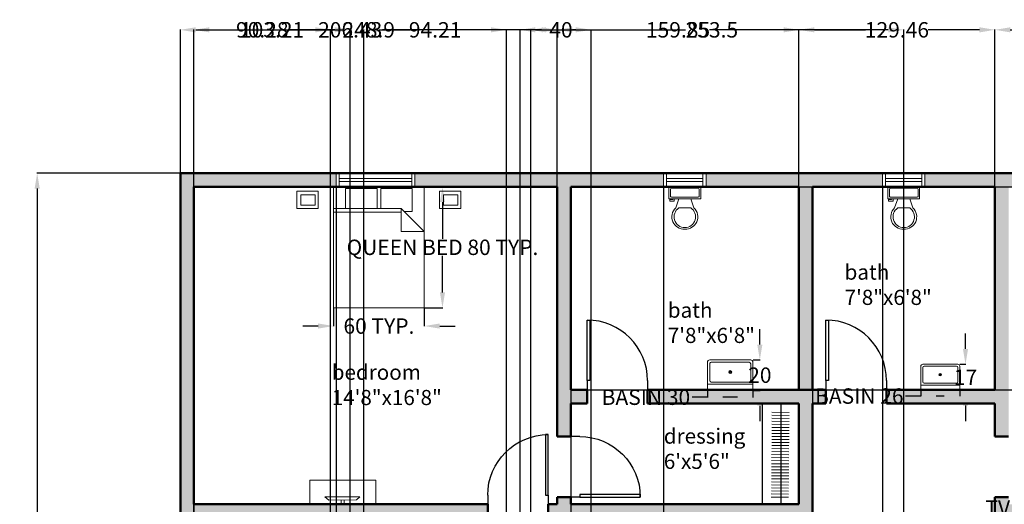
# Model space of a CAD drawing. Units: inches. Extents: x 12496 to 13538, y 6171 to 6892.
# Tile 5 of 6: x 12516 to 13167, y 6572 to 6892. Entities that reach past the tile are written whole.
import ezdxf

# ---------------------------------------------------------------- set-up
doc = ezdxf.new("R2010")
doc.units = ezdxf.units.IN
doc.header["$MEASUREMENT"] = 0
for name, color, linetype, lineweight in [('A-ANNO-DIMS', 2, 'Continuous', 18), ('A-AREA-IDEN', 7, 'Continuous', 25), ('A-DOOR', 3, 'Continuous', 25), ('A-FLOR-CASE', 8, 'Continuous', 25), ('A-FLOR-CASE-PATT', 8, 'Continuous', 13), ('A-FLOR-FIXT', 9, 'Continuous', 18), ('A-FURN', 8, 'Continuous', 18), ('A-GLAZ', 4, 'Continuous', 18), ('A-WALL', 7, 'Continuous', 50)]:
    doc.layers.add(name, color=color, linetype=linetype, lineweight=lineweight)
doc.layers.add('A-WALL-PATT', color=18, linetype='Continuous', lineweight=13, true_color=0x000000)
doc.styles.get("Standard").update_dxf_attribs({"font": 'arial.ttf'})
doc.dimstyles.get("Standard").update_dxf_attribs({"dimtxt": 10.18, "dimasz": 10.18, "dimexe": 0.18, "dimexo": 0.0625, "dimgap": 0.09, "dimtad": 0, "dimtih": 1, "dimtoh": 1, "dimdec": 0, "dimzin": 0, "dimdsep": 46, "dimlunit": 3, "dimtxsty": 'Standard', "dimcen": 0.09, "dimadec": 0, "dimazin": 0, "dimtfac": 1, "dimtdec": 0, "dimtofl": 0, "dimtmove": 0, "dimatfit": 3, "dimfxl": 1, "dimtolj": 1, "dimtzin": 0, "dimarcsym": 0})

# ---------------------------------------------------------------- blocks, each defined once
blk = doc.blocks.new('Bed - Queen')
for p, q in [((0, -80.00003), (0, 0)), ((0, 0), (59.99999, 0)), ((59.99999, 0), (59.99999, -80.00003)), ((7.99999, -1.2), (28.79998, -1.2)), ((7.99999, -14.4), (7.99999, -1.2)), ((28.79998, -1.2), (28.79998, -14.4)), ((31.19999, -1.2), (51.99999, -1.2)), ((31.19999, -14.4), (31.19999, -1.2)), ((51.99999, -1.2), (51.99999, -16.4)), ((0, -14.4), (44.8, -14.4)), ((44.8, -16.8), (0, -16.8)), ((59.99999, -29.6), (44.8, -14.4)), ((44.8, -14.4), (44.8, -29.6)), ((51.99999, -16.4), (46.79936, -16.4)), ((44.8, -29.6), (59.99999, -29.6)), ((59.99999, -80.00003), (0, -80.00003))]:
    blk.add_line(p, q)
blk = doc.blocks.new('*U2')
for p, q in [((0, 0), (0, -6)), ((40, 0), (40, -6))]:
    blk.add_line(p, q)
blk.add_lwpolyline([(0, 0), (0, 40), (1.75, 40), (1.75, 0)], close=True)
blk.add_arc((0, 0), 40, 0, 90)
blk = doc.blocks.new('*U16')
for p, q in [((9.5, -6), (9.5, -2)), ((-10, -8.5), (-8, -8.5)), ((-10, -9.5), (-10, -8.5)), ((-7, -9.5), (-10, -9.5)), ((-8, -8.5), (-8, -8)), ((-7, -8), (-7, -9.5)), ((-4, -8), (-6, -14)), ((4, -8), (6, -14)), ((4, -14), (-4, -14))]:
    blk.add_line(p, q)
blk.add_lwpolyline([(10.5, -8), (10.5, 0), (-10.5, 0), (-10.5, -8)], close=True)
for points in [[(-9.5, -2), (-9.5, -6)], [(8.5, -1), (-8.5, -1)], [(-8.5, -7), (8.5, -7)]]:
    blk.add_lwpolyline(points)
for centre, radius, start, end in [((-8.625, -1.875), 0.8839, 81.8699, 188.1301), ((-8.625, -6.125), 0.8839, 171.869898, 278.1301), ((8.625, -1.875), 0.8839, 351.8699, 98.1301), ((8.625, -6.125), 0.8839, 261.8699, 8.1301), ((-0.4772, -19.9188), 8.0953, 133.01722, 273.38), ((0.0374, -19.8731), 7.127, 124.50543, 269.7), ((-0.0373, -19.8731), 7.127, 270.3, 55.4946), ((0.4773, -19.9188), 8.0953, 266.62, 46.9828)]:
    blk.add_arc(centre, radius, start, end)
blk = doc.blocks.new('Sink-single - 30 in top')
blk.add_line((-15, -3.999996), (15, -3.999996))
for points in [[(-13.5, 0), (13.5, 0)], [(-15, -18.499996), (-15, -1.5)], [(-12.5, -5.499996), (12.5, -5.499996)], [(15, -1.5), (15, -18.499996)], [(-13.5, -17.499996), (-13.5, -6.499996)], [(13.5, -6.499996), (13.5, -17.499996)], [(12.5, -18.499996), (-12.5, -18.499996)], [(13.5, -19.999996), (-13.5, -19.999996)]]:
    blk.add_lwpolyline(points)
for radius in [1, 0.5]:
    blk.add_circle((0, -11.999996), radius)
for centre, radius, start, end in [((-13.5, -1.5), 1.5, 90, 180), ((-12.5, -6.499996), 1, 90, 180), ((12.5, -6.499996), 1, 0, 90), ((13.5, -1.5), 1.5, 0, 90), ((-13.5, -18.499996), 1.5, 180, 270), ((-12.5, -17.499996), 1, 180, 270), ((12.5, -17.499996), 1, 270, 0), ((13.5, -18.499996), 1.5, 270, 0)]:
    blk.add_arc(centre, radius, start, end)
blk = doc.blocks.new('TV-CONSOLE')
for p, q in [((10.88, 32.95), (10.88, 9.78)), ((10.88, 32.95), (12.91, 30.72)), ((12.91, 30.72), (13.04, 12.51)), ((12.98, 22.62), (15.84, 22.62)), ((12.98, 20.62), (15.84, 20.62)), ((10.88, 9.78), (13.04, 12.51))]:
    blk.add_line(p, q)
blk.add_lwpolyline([(15.84, 43.51), (0, 43.51), (0, 0), (15.84, 0)], close=True)
blk = doc.blocks.new('BEDSIDE-TABLE')
for points in [[(0, 11.4), (13.96, 11.4), (13.96, 0), (0, 0)], [(2.55, 8.94), (11.99, 8.94), (11.99, 2.21), (2.55, 2.21)]]:
    blk.add_lwpolyline(points, close=True)
blk = doc.blocks.new('WIN-48IN')
for p, q in [((0, 0), (0, 9)), ((2, 0), (2, 9)), ((50, 0), (50, 9)), ((52, 0), (52, 9)), ((2, 5.5), (50, 5.5)), ((2, 3.5), (50, 3.5))]:
    blk.add_line(p, q)
blk = doc.blocks.new('WIN-24IN')
for p, q in [((0, 0), (0, 9)), ((2, 0), (2, 9)), ((26, 0), (26, 9)), ((28, 0), (28, 9)), ((2, 5.5), (26, 5.5)), ((2, 3.5), (26, 3.5))]:
    blk.add_line(p, q)
blk = doc.blocks.new('*D25')
at = {"layer": 'A-ANNO-DIMS', "color": 0, "lineweight": -2, "transparency": 16777216}
for p, q in [((12783.43, 6781.89), (12795.55, 6781.89)), ((12795.37, 6771.71), (12795.37, 6747.56)), ((12795.37, 6712.07), (12795.37, 6736.23)), ((12783.43, 6701.89), (12795.55, 6701.89))]:
    blk.add_line(p, q, dxfattribs=at)
at = {"layer": 'A-ANNO-DIMS', "color": 0, "transparency": 16777216}
for points in [[(12793.68, 6771.71), (12797.07, 6771.71), (12795.37, 6781.89)], [(12793.68, 6712.07), (12797.07, 6712.07), (12795.37, 6701.89)]]:
    blk.add_solid(points, dxfattribs=at)
at = {"layer": 'Defpoints', "color": 0, "transparency": 16777216}
for p in [(12783.37, 6781.89), (12795.37, 6781.89), (12783.37, 6701.89)]:
    blk.add_point(p, dxfattribs=at)
at = {"layer": 'A-ANNO-DIMS', "color": 0, "transparency": 16777216, "insert": (12795.37, 6741.89), "char_height": 10.18, "attachment_point": 5}
blk.add_mtext('\\A1;QUEEN BED 80 TYP.', dxfattribs=at)
blk = doc.blocks.new('*D26')
at = {"layer": 'A-ANNO-DIMS', "color": 0, "lineweight": -2, "transparency": 16777216}
for p, q in [((12723.37, 6701.83), (12723.37, 6689.71)), ((12783.37, 6701.83), (12783.37, 6689.71)), ((12713.19, 6689.89), (12703.01, 6689.89)), ((12793.55, 6689.89), (12803.73, 6689.89))]:
    blk.add_line(p, q, dxfattribs=at)
at = {"layer": 'A-ANNO-DIMS', "color": 0, "transparency": 16777216}
for points in [[(12713.19, 6691.59), (12713.19, 6688.2), (12723.37, 6689.89)], [(12793.55, 6691.59), (12793.55, 6688.2), (12783.37, 6689.89)]]:
    blk.add_solid(points, dxfattribs=at)
at = {"layer": 'Defpoints', "color": 0, "transparency": 16777216}
for p in [(12723.37, 6701.89), (12783.37, 6701.89), (12783.37, 6689.89)]:
    blk.add_point(p, dxfattribs=at)
at = {"layer": 'A-ANNO-DIMS', "color": 0, "transparency": 16777216, "insert": (12753.37, 6689.89), "char_height": 10.18, "attachment_point": 5}
blk.add_mtext('\\A1;60 TYP.', dxfattribs=at)
blk = doc.blocks.new('*D29')
at = {"layer": 'A-ANNO-DIMS', "color": 0, "lineweight": -2, "transparency": 16777216}
for p, q in [((13303.55, 6569.73), (13293.37, 6569.73)), ((13303.55, 6563.27), (13303.55, 6569.91)), ((13336.87, 6569.73), (13313.73, 6569.73)), ((13347.05, 6563.27), (13347.05, 6569.91))]:
    blk.add_line(p, q, dxfattribs=at)
at = {"layer": 'A-ANNO-DIMS', "color": 0, "transparency": 16777216}
for points in [[(13313.73, 6571.43), (13313.73, 6568.03), (13303.55, 6569.73)], [(13336.87, 6571.43), (13336.87, 6568.03), (13347.05, 6569.73)]]:
    blk.add_solid(points, dxfattribs=at)
at = {"layer": 'Defpoints', "color": 0, "transparency": 16777216}
for p in [(13303.55, 6569.73), (13303.55, 6563.2), (13347.05, 6563.2)]:
    blk.add_point(p, dxfattribs=at)
at = {"layer": 'A-ANNO-DIMS', "color": 0, "transparency": 16777216, "insert": (13220.56, 6569.73), "char_height": 10.18, "attachment_point": 5}
blk.add_mtext('\\A1;TV CONSOLE 44 TYP.', dxfattribs=at)
blk = doc.blocks.new('*D39')
at = {"layer": 'A-ANNO-DIMS', "color": 0, "lineweight": -2, "transparency": 16777216}
for p, q in [((12970.42, 6642.9), (12960.24, 6642.9)), ((12970.42, 6647.36), (12970.42, 6642.72)), ((12990.36, 6642.9), (12980.6, 6642.9)), ((13000.54, 6647.36), (13000.54, 6642.72))]:
    blk.add_line(p, q, dxfattribs=at)
at = {"layer": 'A-ANNO-DIMS', "color": 0, "transparency": 16777216}
for points in [[(12980.6, 6644.6), (12980.6, 6641.21), (12970.42, 6642.9)], [(12990.36, 6644.6), (12990.36, 6641.21), (13000.54, 6642.9)]]:
    blk.add_solid(points, dxfattribs=at)
at = {"layer": 'Defpoints', "color": 0, "transparency": 16777216}
for p in [(12970.42, 6647.42), (12970.42, 6642.9), (13000.54, 6647.42)]:
    blk.add_point(p, dxfattribs=at)
at = {"layer": 'A-ANNO-DIMS', "color": 0, "transparency": 16777216, "insert": (12929.78, 6642.9), "char_height": 10.18, "attachment_point": 5}
blk.add_mtext('\\A1;BASIN 30', dxfattribs=at)
blk = doc.blocks.new('*D40')
at = {"layer": 'A-ANNO-DIMS', "color": 0, "lineweight": -2, "transparency": 16777216}
for p, q in [((13005.06, 6677.68), (13005.06, 6687.86)), ((13000.6, 6667.5), (13005.24, 6667.5)), ((13000.6, 6647.42), (13005.24, 6647.42)), ((13005.06, 6637.24), (13005.06, 6627.06))]:
    blk.add_line(p, q, dxfattribs=at)
at = {"layer": 'A-ANNO-DIMS', "color": 0, "transparency": 16777216}
for points in [[(13003.36, 6677.68), (13006.75, 6677.68), (13005.06, 6667.5)], [(13003.36, 6637.24), (13006.75, 6637.24), (13005.06, 6647.42)]]:
    blk.add_solid(points, dxfattribs=at)
at = {"layer": 'Defpoints', "color": 0, "transparency": 16777216}
for p in [(13000.54, 6667.5), (13000.54, 6647.42), (13005.06, 6647.42)]:
    blk.add_point(p, dxfattribs=at)
at = {"layer": 'A-ANNO-DIMS', "color": 0, "transparency": 16777216, "insert": (13005.06, 6657.46), "char_height": 10.18, "attachment_point": 5}
blk.add_mtext('\\A1;20', dxfattribs=at)
blk = doc.blocks.new('*D41')
at = {"layer": 'A-ANNO-DIMS', "color": 0, "lineweight": -2, "transparency": 16777216}
for p, q in [((13111.44, 6643.67), (13101.26, 6643.67)), ((13111.44, 6647.46), (13111.44, 6643.49)), ((13126.92, 6643.67), (13121.62, 6643.67)), ((13137.1, 6647.46), (13137.1, 6643.49))]:
    blk.add_line(p, q, dxfattribs=at)
at = {"layer": 'A-ANNO-DIMS', "color": 0, "transparency": 16777216}
for points in [[(13121.62, 6645.37), (13121.62, 6641.98), (13111.44, 6643.67)], [(13126.92, 6645.37), (13126.92, 6641.98), (13137.1, 6643.67)]]:
    blk.add_solid(points, dxfattribs=at)
at = {"layer": 'Defpoints', "color": 0, "transparency": 16777216}
for p in [(13111.44, 6647.52), (13111.44, 6643.67), (13137.1, 6647.52)]:
    blk.add_point(p, dxfattribs=at)
at = {"layer": 'A-ANNO-DIMS', "color": 0, "transparency": 16777216, "insert": (13070.79, 6643.67), "char_height": 10.18, "attachment_point": 5}
blk.add_mtext('\\A1;BASIN 26', dxfattribs=at)
blk = doc.blocks.new('*D42')
at = {"layer": 'A-ANNO-DIMS', "color": 0, "lineweight": -2, "transparency": 16777216}
for p, q in [((13140.95, 6674.81), (13140.95, 6684.99)), ((13137.16, 6664.63), (13141.13, 6664.63)), ((13137.16, 6647.52), (13141.13, 6647.52)), ((13140.95, 6637.34), (13140.95, 6627.16))]:
    blk.add_line(p, q, dxfattribs=at)
at = {"layer": 'A-ANNO-DIMS', "color": 0, "transparency": 16777216}
for points in [[(13139.25, 6674.81), (13142.65, 6674.81), (13140.95, 6664.63)], [(13139.25, 6637.34), (13142.65, 6637.34), (13140.95, 6647.52)]]:
    blk.add_solid(points, dxfattribs=at)
at = {"layer": 'Defpoints', "color": 0, "transparency": 16777216}
for p in [(13137.1, 6664.63), (13137.1, 6647.52), (13140.95, 6647.52)]:
    blk.add_point(p, dxfattribs=at)
at = {"layer": 'A-ANNO-DIMS', "color": 0, "transparency": 16777216, "insert": (13140.95, 6656.08), "char_height": 10.18, "attachment_point": 5}
blk.add_mtext('\\A1;17', dxfattribs=at)
blk = doc.blocks.new('*D60')
at = {"layer": 'A-ANNO-DIMS', "color": 0, "lineweight": -2, "transparency": 16777216}
for p, q in [((12622.11, 6790.89), (12527.4, 6790.89)), ((12527.58, 6780.71), (12527.58, 6511.18)), ((12527.58, 6231.07), (12527.58, 6500.61)), ((12622.11, 6220.89), (12527.4, 6220.89))]:
    blk.add_line(p, q, dxfattribs=at)
at = {"layer": 'A-ANNO-DIMS', "color": 0, "transparency": 16777216}
for points in [[(12525.88, 6780.71), (12529.28, 6780.71), (12527.58, 6790.89)], [(12525.88, 6231.07), (12529.28, 6231.07), (12527.58, 6220.89)]]:
    blk.add_solid(points, dxfattribs=at)
at = {"layer": 'Defpoints', "color": 0, "transparency": 16777216}
for p in [(12527.58, 6790.89), (12622.17, 6790.89), (12622.17, 6220.89)]:
    blk.add_point(p, dxfattribs=at)
at = {"layer": 'A-ANNO-DIMS', "color": 0, "transparency": 16777216, "insert": (12527.58, 6505.89), "char_height": 10.18, "attachment_point": 5}
blk.add_mtext('\\A1;570', dxfattribs=at)
blk = doc.blocks.new('*D61')
at = {"layer": 'A-ANNO-DIMS', "color": 0, "lineweight": -2, "transparency": 16777216}
for p, q in [((12622.17, 6790.96), (12622.17, 6885.67)), ((12632.35, 6885.49), (12729.26, 6885.49)), ((12860.89, 6885.49), (12763.99, 6885.49)), ((12871.07, 6781.96), (12871.07, 6885.67))]:
    blk.add_line(p, q, dxfattribs=at)
at = {"layer": 'A-ANNO-DIMS', "color": 0, "transparency": 16777216}
for points in [[(12632.35, 6887.18), (12632.35, 6883.79), (12622.17, 6885.49)], [(12860.89, 6887.18), (12860.89, 6883.79), (12871.07, 6885.49)]]:
    blk.add_solid(points, dxfattribs=at)
at = {"layer": 'Defpoints', "color": 0, "transparency": 16777216}
for p in [(12871.07, 6885.49), (12622.17, 6790.89), (12871.07, 6781.89)]:
    blk.add_point(p, dxfattribs=at)
at = {"layer": 'A-ANNO-DIMS', "color": 0, "transparency": 16777216, "insert": (12746.62, 6885.49), "char_height": 10.18, "attachment_point": 5}
blk.add_mtext('\\A1;248.9', dxfattribs=at)
blk = doc.blocks.new('*D62')
at = {"layer": 'A-ANNO-DIMS', "color": 0, "lineweight": -2, "transparency": 16777216}
for p, q in [((12871.07, 6781.96), (12871.07, 6885.67)), ((12881.25, 6885.49), (12930.22, 6885.49)), ((13020.74, 6885.49), (12971.78, 6885.49)), ((13030.92, 6781.96), (13030.92, 6885.67))]:
    blk.add_line(p, q, dxfattribs=at)
at = {"layer": 'A-ANNO-DIMS', "color": 0, "transparency": 16777216}
for points in [[(12881.25, 6887.18), (12881.25, 6883.79), (12871.07, 6885.49)], [(13020.74, 6887.18), (13020.74, 6883.79), (13030.92, 6885.49)]]:
    blk.add_solid(points, dxfattribs=at)
at = {"layer": 'Defpoints', "color": 0, "transparency": 16777216}
for p in [(13030.92, 6885.49), (12871.07, 6781.89), (13030.92, 6781.89)]:
    blk.add_point(p, dxfattribs=at)
at = {"layer": 'A-ANNO-DIMS', "color": 0, "transparency": 16777216, "insert": (12951, 6885.49), "char_height": 10.18, "attachment_point": 5}
blk.add_mtext('\\A1;159.85', dxfattribs=at)
blk = doc.blocks.new('*D63')
at = {"layer": 'A-ANNO-DIMS', "color": 0, "lineweight": -2, "transparency": 16777216}
for p, q in [((13030.92, 6781.96), (13030.92, 6885.67)), ((13041.1, 6885.49), (13074.91, 6885.49)), ((13150.2, 6885.49), (13116.39, 6885.49)), ((13160.38, 6781.96), (13160.38, 6885.67))]:
    blk.add_line(p, q, dxfattribs=at)
at = {"layer": 'A-ANNO-DIMS', "color": 0, "transparency": 16777216}
for points in [[(13041.1, 6887.18), (13041.1, 6883.79), (13030.92, 6885.49)], [(13150.2, 6887.18), (13150.2, 6883.79), (13160.38, 6885.49)]]:
    blk.add_solid(points, dxfattribs=at)
at = {"layer": 'Defpoints', "color": 0, "transparency": 16777216}
for p in [(13160.38, 6885.49), (13030.92, 6781.89), (13160.38, 6781.89)]:
    blk.add_point(p, dxfattribs=at)
at = {"layer": 'A-ANNO-DIMS', "color": 0, "transparency": 16777216, "insert": (13095.65, 6885.49), "char_height": 10.18, "attachment_point": 5}
blk.add_mtext('\\A1;129.46', dxfattribs=at)
blk = doc.blocks.new('*D64')
at = {"layer": 'A-ANNO-DIMS', "color": 0, "lineweight": -2, "transparency": 16777216}
for p, q in [((13160.38, 6781.96), (13160.38, 6885.67)), ((13170.56, 6885.49), (13280.36, 6885.49)), ((13432.85, 6885.49), (13323.05, 6885.49)), ((13443.03, 6790.96), (13443.03, 6885.67))]:
    blk.add_line(p, q, dxfattribs=at)
at = {"layer": 'A-ANNO-DIMS', "color": 0, "transparency": 16777216}
for points in [[(13170.56, 6887.18), (13170.56, 6883.79), (13160.38, 6885.49)], [(13432.85, 6887.18), (13432.85, 6883.79), (13443.03, 6885.49)]]:
    blk.add_solid(points, dxfattribs=at)
at = {"layer": 'Defpoints', "color": 0, "transparency": 16777216}
for p in [(13443.03, 6885.49), (13443.03, 6790.89), (13160.38, 6781.89)]:
    blk.add_point(p, dxfattribs=at)
at = {"layer": 'A-ANNO-DIMS', "color": 0, "transparency": 16777216, "insert": (13301.7, 6885.49), "char_height": 10.18, "attachment_point": 5}
blk.add_mtext('\\A1;282.65', dxfattribs=at)
blk = doc.blocks.new('*D65')
at = {"layer": 'A-ANNO-DIMS', "color": 0, "lineweight": -2, "transparency": 16777216}
for p, q in [((12631.17, 6229.96), (12631.17, 6885.67)), ((12641.35, 6885.49), (12713.08, 6885.49)), ((12827.42, 6885.49), (12755.7, 6885.49)), ((12837.6, 6229.96), (12837.6, 6885.67))]:
    blk.add_line(p, q, dxfattribs=at)
at = {"layer": 'A-ANNO-DIMS', "color": 0, "transparency": 16777216}
for points in [[(12641.35, 6887.18), (12641.35, 6883.79), (12631.17, 6885.49)], [(12827.42, 6887.18), (12827.42, 6883.79), (12837.6, 6885.49)]]:
    blk.add_solid(points, dxfattribs=at)
at = {"layer": 'Defpoints', "color": 0, "transparency": 16777216}
for p in [(12837.6, 6885.49), (12631.17, 6229.89), (12837.6, 6229.89)]:
    blk.add_point(p, dxfattribs=at)
at = {"layer": 'A-ANNO-DIMS', "color": 0, "transparency": 16777216, "insert": (12734.39, 6885.49), "char_height": 10.18, "attachment_point": 5}
blk.add_mtext('\\A1;206.43', dxfattribs=at)
blk = doc.blocks.new('*D66')
at = {"layer": 'A-ANNO-DIMS', "color": 0, "lineweight": -2, "transparency": 16777216}
for p, q in [((12846.6, 6312.58), (12846.6, 6885.67)), ((12856.78, 6885.49), (12955.96, 6885.49)), ((13089.92, 6885.49), (12990.74, 6885.49)), ((13100.1, 6312.58), (13100.1, 6885.67))]:
    blk.add_line(p, q, dxfattribs=at)
at = {"layer": 'A-ANNO-DIMS', "color": 0, "transparency": 16777216}
for points in [[(12856.78, 6887.18), (12856.78, 6883.79), (12846.6, 6885.49)], [(13089.92, 6887.18), (13089.92, 6883.79), (13100.1, 6885.49)]]:
    blk.add_solid(points, dxfattribs=at)
at = {"layer": 'Defpoints', "color": 0, "transparency": 16777216}
for p in [(13100.1, 6885.49), (12846.6, 6312.52), (13100.1, 6312.52)]:
    blk.add_point(p, dxfattribs=at)
at = {"layer": 'A-ANNO-DIMS', "color": 0, "transparency": 16777216, "insert": (12973.35, 6885.49), "char_height": 10.18, "attachment_point": 5}
blk.add_mtext('\\A1;253.5', dxfattribs=at)
blk = doc.blocks.new('*D70')
at = {"layer": 'A-ANNO-DIMS', "color": 0, "lineweight": -2, "transparency": 16777216}
for p, q in [((12880.13, 6781.89), (13486.8, 6781.89)), ((13486.62, 6771.71), (13486.62, 6720.17)), ((13486.62, 6658.04), (13486.62, 6709.59)), ((12880.13, 6647.86), (13486.8, 6647.86))]:
    blk.add_line(p, q, dxfattribs=at)
at = {"layer": 'A-ANNO-DIMS', "color": 0, "transparency": 16777216}
for points in [[(13484.92, 6771.71), (13488.32, 6771.71), (13486.62, 6781.89)], [(13484.92, 6658.04), (13488.32, 6658.04), (13486.62, 6647.86)]]:
    blk.add_solid(points, dxfattribs=at)
at = {"layer": 'Defpoints', "color": 0, "transparency": 16777216}
for p in [(12880.07, 6781.89), (12880.07, 6647.86), (13486.62, 6647.86)]:
    blk.add_point(p, dxfattribs=at)
at = {"layer": 'A-ANNO-DIMS', "color": 0, "transparency": 16777216, "insert": (13486.62, 6714.88), "char_height": 10.18, "attachment_point": 5}
blk.add_mtext('\\A1;134.03', dxfattribs=at)
blk = doc.blocks.new('*D73')
at = {"layer": 'A-ANNO-DIMS', "color": 0, "lineweight": -2, "transparency": 16777216}
for p, q in [((12631.17, 6393.87), (12631.17, 6885.67)), ((12641.35, 6885.49), (12663.02, 6885.49)), ((12724.21, 6885.49), (12702.54, 6885.49)), ((12734.39, 6393.87), (12734.39, 6885.67))]:
    blk.add_line(p, q, dxfattribs=at)
at = {"layer": 'A-ANNO-DIMS', "color": 0, "transparency": 16777216}
for points in [[(12641.35, 6887.18), (12641.35, 6883.79), (12631.17, 6885.49)], [(12724.21, 6887.18), (12724.21, 6883.79), (12734.39, 6885.49)]]:
    blk.add_solid(points, dxfattribs=at)
at = {"layer": 'Defpoints', "color": 0, "transparency": 16777216}
for p in [(12734.39, 6885.49), (12631.17, 6393.81), (12734.39, 6393.81)]:
    blk.add_point(p, dxfattribs=at)
at = {"layer": 'A-ANNO-DIMS', "color": 0, "transparency": 16777216, "insert": (12682.78, 6885.49), "char_height": 10.18, "attachment_point": 5}
blk.add_mtext('\\A1;103.21', dxfattribs=at)
blk = doc.blocks.new('*D75')
at = {"layer": 'A-ANNO-DIMS', "color": 0, "lineweight": -2, "transparency": 16777216}
for p, q in [((12631.17, 6563.27), (12631.17, 6885.67)), ((12641.35, 6885.49), (12659.04, 6885.49)), ((12711.27, 6885.49), (12693.59, 6885.49)), ((12721.45, 6563.27), (12721.45, 6885.67))]:
    blk.add_line(p, q, dxfattribs=at)
at = {"layer": 'A-ANNO-DIMS', "color": 0, "transparency": 16777216}
for points in [[(12641.35, 6887.18), (12641.35, 6883.79), (12631.17, 6885.49)], [(12711.27, 6887.18), (12711.27, 6883.79), (12721.45, 6885.49)]]:
    blk.add_solid(points, dxfattribs=at)
at = {"layer": 'Defpoints', "color": 0, "transparency": 16777216}
for p in [(12721.45, 6885.49), (12631.17, 6563.2), (12721.45, 6563.2)]:
    blk.add_point(p, dxfattribs=at)
at = {"layer": 'A-ANNO-DIMS', "color": 0, "transparency": 16777216, "insert": (12676.31, 6885.49), "char_height": 10.18, "attachment_point": 5}
blk.add_mtext('\\A1;90.28', dxfattribs=at)
blk = doc.blocks.new('*D80')
at = {"layer": 'A-ANNO-DIMS', "color": 0, "lineweight": -2, "transparency": 16777216}
for p, q in [((12631.17, 6781.83), (12631.17, 6177.12)), ((12725.12, 6781.83), (12725.12, 6177.12)), ((12641.35, 6177.3), (12660.84, 6177.3)), ((12714.94, 6177.3), (12695.45, 6177.3))]:
    blk.add_line(p, q, dxfattribs=at)
at = {"layer": 'A-ANNO-DIMS', "color": 0, "transparency": 16777216}
for points in [[(12641.35, 6179), (12641.35, 6175.6), (12631.17, 6177.3)], [(12714.94, 6179), (12714.94, 6175.6), (12725.12, 6177.3)]]:
    blk.add_solid(points, dxfattribs=at)
at = {"layer": 'Defpoints', "color": 0, "transparency": 16777216}
for p in [(12631.17, 6781.89), (12725.12, 6781.89), (12725.12, 6177.3)]:
    blk.add_point(p, dxfattribs=at)
at = {"layer": 'A-ANNO-DIMS', "color": 0, "transparency": 16777216, "insert": (12678.15, 6177.3), "char_height": 10.18, "attachment_point": 5}
blk.add_mtext('\\A1;93.95', dxfattribs=at)
blk = doc.blocks.new('*D81')
at = {"layer": 'A-ANNO-DIMS', "color": 0, "lineweight": -2, "transparency": 16777216}
for p, q in [((12880.07, 6781.83), (12880.07, 6177.12)), ((12941.5, 6781.83), (12941.5, 6177.12)), ((12890.25, 6177.3), (12893.54, 6177.3)), ((12931.32, 6177.3), (12928.02, 6177.3))]:
    blk.add_line(p, q, dxfattribs=at)
at = {"layer": 'A-ANNO-DIMS', "color": 0, "transparency": 16777216}
for points in [[(12890.25, 6179), (12890.25, 6175.6), (12880.07, 6177.3)], [(12931.32, 6179), (12931.32, 6175.6), (12941.5, 6177.3)]]:
    blk.add_solid(points, dxfattribs=at)
at = {"layer": 'Defpoints', "color": 0, "transparency": 16777216}
for p in [(12880.07, 6781.89), (12941.5, 6781.89), (12941.5, 6177.3)]:
    blk.add_point(p, dxfattribs=at)
at = {"layer": 'A-ANNO-DIMS', "color": 0, "transparency": 16777216, "insert": (12910.78, 6177.3), "char_height": 10.18, "attachment_point": 5}
blk.add_mtext('\\A1;61.42', dxfattribs=at)
blk = doc.blocks.new('*D82')
at = {"layer": 'A-ANNO-DIMS', "color": 0, "lineweight": -2, "transparency": 16777216}
for p, q in [((13039.92, 6781.83), (13039.92, 6177.12)), ((13086.15, 6781.83), (13086.15, 6177.12)), ((13029.74, 6177.3), (13019.56, 6177.3)), ((13096.33, 6177.3), (13106.51, 6177.3))]:
    blk.add_line(p, q, dxfattribs=at)
at = {"layer": 'A-ANNO-DIMS', "color": 0, "transparency": 16777216}
for points in [[(13029.74, 6179), (13029.74, 6175.6), (13039.92, 6177.3)], [(13096.33, 6179), (13096.33, 6175.6), (13086.15, 6177.3)]]:
    blk.add_solid(points, dxfattribs=at)
at = {"layer": 'Defpoints', "color": 0, "transparency": 16777216}
for p in [(13039.92, 6781.89), (13086.15, 6781.89), (13086.15, 6177.3)]:
    blk.add_point(p, dxfattribs=at)
at = {"layer": 'A-ANNO-DIMS', "color": 0, "transparency": 16777216, "insert": (13063.03, 6177.3), "char_height": 10.18, "attachment_point": 5}
blk.add_mtext('\\A1;46.23', dxfattribs=at)
blk = doc.blocks.new('*D84')
at = {"layer": 'A-ANNO-DIMS', "color": 0, "lineweight": -2, "transparency": 16777216}
for p, q in [((12853.64, 6312.58), (12853.64, 6885.67)), ((12863.82, 6885.49), (12866.07, 6885.49)), ((12883.46, 6885.49), (12881.21, 6885.49)), ((12893.64, 6312.58), (12893.64, 6885.67))]:
    blk.add_line(p, q, dxfattribs=at)
at = {"layer": 'A-ANNO-DIMS', "color": 0, "transparency": 16777216}
for points in [[(12863.82, 6887.18), (12863.82, 6883.79), (12853.64, 6885.49)], [(12883.46, 6887.18), (12883.46, 6883.79), (12893.64, 6885.49)]]:
    blk.add_solid(points, dxfattribs=at)
at = {"layer": 'Defpoints', "color": 0, "transparency": 16777216}
for p in [(12893.64, 6885.49), (12853.64, 6312.52), (12893.64, 6312.52)]:
    blk.add_point(p, dxfattribs=at)
at = {"layer": 'A-ANNO-DIMS', "color": 0, "transparency": 16777216, "insert": (12873.64, 6885.49), "char_height": 10.18, "attachment_point": 5}
blk.add_mtext('\\A1;40', dxfattribs=at)
blk = doc.blocks.new('*D85')
at = {"layer": 'A-ANNO-DIMS', "color": 0, "lineweight": -2, "transparency": 16777216}
for p, q in [((12743.39, 6402.87), (12743.39, 6885.67)), ((12753.57, 6885.49), (12774.21, 6885.49)), ((12827.42, 6885.49), (12806.78, 6885.49)), ((12837.6, 6402.87), (12837.6, 6885.67))]:
    blk.add_line(p, q, dxfattribs=at)
at = {"layer": 'A-ANNO-DIMS', "color": 0, "transparency": 16777216}
for points in [[(12753.57, 6887.18), (12753.57, 6883.79), (12743.39, 6885.49)], [(12827.42, 6887.18), (12827.42, 6883.79), (12837.6, 6885.49)]]:
    blk.add_solid(points, dxfattribs=at)
at = {"layer": 'Defpoints', "color": 0, "transparency": 16777216}
for p in [(12837.6, 6885.49), (12743.39, 6402.81), (12837.6, 6402.81)]:
    blk.add_point(p, dxfattribs=at)
at = {"layer": 'A-ANNO-DIMS', "color": 0, "transparency": 16777216, "insert": (12790.5, 6885.49), "char_height": 10.18, "attachment_point": 5}
blk.add_mtext('\\A1;94.21', dxfattribs=at)

msp = doc.modelspace()

# ---------------------------------------------------------------- hatches: boundary and pattern name
at = {"layer": 'A-FLOR-CASE-PATT'}
h = msp.add_hatch(dxfattribs=at)
h.set_pattern_fill('ANSI31', color=256, scale=16, angle=134.51908, style=0)
h.paths.add_polyline_path([(13012.6228, 6576.4479), (13024.0245, 6576.3522), (13024.5113, 6634.3501), (13013.1096, 6634.4458)])
at = {"layer": 'A-WALL-PATT'}
h = msp.add_hatch(color=256, dxfattribs=at)
h.dxf.hatch_style = 1
h.paths.add_polyline_path([(12631.1731, 6781.8943), (12725.1219, 6781.8943), (12725.1219, 6790.8943), (12622.1731, 6790.8943), (12622.1731, 6551.6486), (12631.1731, 6551.6486), (12631.1731, 6563.2028), (12825.2657, 6563.2028), (12825.2657, 6572.2028), (12631.1731, 6572.2028)])
h.paths.add_polyline_path([(12941.4956, 6790.8943), (12777.1219, 6790.8943), (12777.1219, 6781.8943), (12871.0706, 6781.8943), (12871.0706, 6616.9323), (12880.0706, 6616.9323), (12880.0706, 6638.8628), (12890.9211, 6638.8628), (12890.9211, 6647.8628), (12880.0706, 6647.8628), (12880.0706, 6781.8943), (12941.4956, 6781.8943)])
h.paths.add_polyline_path([(13039.9206, 6781.8943), (13086.1485, 6781.8943), (13086.1485, 6790.8943), (12969.4956, 6790.8943), (12969.4956, 6781.8943), (13030.9206, 6781.8943), (13030.9206, 6647.8628), (13039.9206, 6647.8628)])
h.paths.add_polyline_path([(13275.7025, 6790.8943), (13114.1485, 6790.8943), (13114.1485, 6781.8943), (13160.3765, 6781.8943), (13160.3765, 6647.8628), (13088.7069, 6647.8628), (13088.7069, 6638.8628), (13160.3765, 6638.8628), (13160.3765, 6616.9323), (13169.3765, 6616.9323), (13169.3765, 6781.8943), (13275.7025, 6781.8943)])
h = msp.add_hatch(color=256, dxfattribs=at)
h.dxf.hatch_style = 1
h.paths.add_polyline_path([(13443.0285, 6790.8943), (13327.7025, 6790.8943), (13327.7025, 6781.8943), (13434.0285, 6781.8943), (13434.0285, 6572.2028), (13169.3765, 6572.2028), (13169.3765, 6576.9323), (13160.3765, 6576.9323), (13160.3765, 6563.2028), (13163.811, 6563.2028), (13163.811, 6559.305), (13172.811, 6559.305), (13172.811, 6563.2028), (13434.0285, 6563.2028), (13434.0285, 6402.794), (13331.4198, 6402.794), (13331.4198, 6393.8103), (13434.0285, 6393.8103), (13434.0285, 6220.8943), (13443.0285, 6220.8943)])
h.paths.add_polyline_path([(13172.811, 6519.305), (13163.811, 6519.305), (13163.811, 6402.8103), (12944.6655, 6402.8103), (12944.6655, 6393.8103), (13100.0985, 6393.8103), (13100.0985, 6312.5223), (13035.7682, 6312.5223), (13035.7682, 6303.5223), (13109.0985, 6303.5223), (13109.0985, 6393.8103), (13279.4198, 6393.8103), (13279.4198, 6402.8103), (13172.811, 6402.8103)])
h.paths.add_polyline_path([(13109.0985, 6229.8943), (12846.603, 6229.8943), (12846.603, 6303.5223), (12853.6371, 6303.5223), (12853.6371, 6312.5223), (12846.603, 6312.5223), (12846.603, 6393.8103), (12872.7237, 6393.8103), (12872.7237, 6402.8103), (12846.603, 6402.8103), (12837.603, 6402.8103), (12837.603, 6229.8943), (12760.3881, 6229.8943), (12760.3881, 6220.8943), (13109.0985, 6220.8943)])
h.paths.add_polyline_path([(12708.3881, 6229.8943), (12631.1731, 6229.8943), (12631.1731, 6336.5598), (12702.8967, 6336.5598), (12702.8967, 6345.5598), (12631.1731, 6345.5598), (12631.1731, 6355.6851), (12622.1731, 6355.6851), (12622.1731, 6220.8943), (12708.3881, 6220.8943)])
h.paths.add_polyline_path([(12743.3881, 6402.8103), (12631.1731, 6402.8103), (12631.1731, 6523.6486), (12622.1731, 6523.6486), (12622.1731, 6383.6851), (12631.1731, 6383.6851), (12631.1731, 6393.8103), (12734.3881, 6393.8103), (12734.3881, 6345.5598), (12731.8151, 6345.5598), (12731.8151, 6336.5598), (12734.3881, 6336.5598), (12743.3881, 6336.5598)])
h.paths.add_polyline_path([(13039.9206, 6572.2028), (13039.9206, 6638.8628), (13048.7069, 6638.8628), (13048.7069, 6647.8628), (13039.9206, 6647.8628), (12930.9211, 6647.8628), (12930.9211, 6638.8628), (13030.9206, 6638.8628), (13030.9206, 6572.2028), (12880.0706, 6572.2028), (12880.0706, 6576.9323), (12871.0706, 6576.9323), (12871.0706, 6572.2028), (12865.2657, 6572.2028), (12865.2657, 6563.2028), (13039.9206, 6563.2028)])
h.paths.add_polyline_path([(13039.9206, 6781.8943), (13086.1485, 6781.8943), (13086.1485, 6790.8943), (12969.4956, 6790.8943), (12969.4956, 6781.8943), (13030.9206, 6781.8943), (13030.9206, 6647.8628), (13039.9206, 6647.8628)])
h.paths.add_polyline_path([(13169.3765, 6781.8943), (13275.7025, 6781.8943), (13275.7025, 6790.8943), (13114.1485, 6790.8943), (13114.1485, 6781.8943), (13160.3765, 6781.8943), (13160.3765, 6647.8628), (13088.7069, 6647.8628), (13088.7069, 6638.8628), (13160.3765, 6638.8628), (13160.3765, 6616.9323), (13169.3765, 6616.9323)])

# ---------------------------------------------------------------- linework, layer by layer
at = {"layer": 'A-FLOR-CASE'}
for p, q in [((13006.6054, 6638.8628), (13006.6054, 6572.2028)), ((13018.9711, 6638.8628), (13018.9711, 6572.2028))]:
    msp.add_line(p, q, dxfattribs=at)
at = {"layer": 'A-WALL'}
for p, q in [((12622.1731, 6220.8943), (12622.1731, 6790.8943)), ((12622.1731, 6790.8943), (13443.0285, 6790.8943)), ((12631.1731, 6781.8943), (12871.0706, 6781.8943)), ((12631.1731, 6572.2028), (12631.1731, 6781.8943)), ((12871.0706, 6616.9323), (12871.0706, 6781.8943)), ((12880.0706, 6647.8628), (12880.0706, 6781.8943)), ((12880.0706, 6781.8943), (13030.9206, 6781.8943)), ((13030.9206, 6647.8628), (13030.9206, 6781.8943)), ((13039.9206, 6781.8943), (13160.3765, 6781.8943)), ((13039.9206, 6647.8628), (13039.9206, 6781.8943)), ((13160.3765, 6647.8628), (13160.3765, 6781.8943)), ((12880.0706, 6647.8628), (12890.9211, 6647.8628)), ((12890.9211, 6647.8628), (12890.9211, 6638.8628)), ((12930.9211, 6647.8628), (12930.9211, 6638.8628)), ((12930.9211, 6647.8628), (13039.9206, 6647.8628)), ((13039.9206, 6647.8628), (13048.7069, 6647.8628)), ((13048.7069, 6647.8628), (13048.7069, 6638.8628)), ((13088.7069, 6647.8628), (13088.7069, 6638.8628)), ((13088.7069, 6647.8628), (13160.3765, 6647.8628)), ((12880.0706, 6638.8628), (12890.9211, 6638.8628)), ((12880.0706, 6616.9323), (12880.0706, 6638.8628)), ((12930.9211, 6638.8628), (13030.9206, 6638.8628)), ((13030.9206, 6572.2028), (13030.9206, 6638.8628)), ((13039.9206, 6572.2028), (13039.9206, 6638.8628)), ((13039.9206, 6638.8628), (13048.7069, 6638.8628)), ((13088.7069, 6638.8628), (13160.3765, 6638.8628)), ((13160.3765, 6616.9323), (13160.3765, 6638.8628)), ((12880.0706, 6616.9323), (12871.0706, 6616.9323)), ((13169.3765, 6616.9323), (13160.3765, 6616.9323)), ((12631.1731, 6572.2028), (12825.2657, 6572.2028)), ((12825.2657, 6572.2028), (12825.2657, 6563.2028)), ((12865.2657, 6572.2028), (12865.2657, 6563.2028)), ((12865.2657, 6572.2028), (12871.0706, 6572.2028)), ((12871.0706, 6572.2028), (12871.0706, 6576.9323)), ((12880.0706, 6576.9323), (12871.0706, 6576.9323)), ((12880.0706, 6572.2028), (12880.0706, 6576.9323)), ((12880.0706, 6572.2028), (13030.9206, 6572.2028)), ((13039.9206, 6563.2028), (13039.9206, 6572.2028)), ((13160.3765, 6563.2028), (13160.3765, 6576.9323)), ((13169.3765, 6576.9323), (13160.3765, 6576.9323))]:
    msp.add_line(p, q, dxfattribs=at)

# ---------------------------------------------------------------- block references
at = {"layer": 'A-DOOR'}
for p in [(12890.9211, 6653.8628), (13048.7069, 6653.8628)]:
    msp.add_blockref('*U2', p, dxfattribs=at)
at = {"layer": 'A-DOOR', "xscale": -1}
msp.add_blockref('*U2', (12865.2657, 6578.2028), dxfattribs=at)
at = {"layer": 'A-DOOR', "xscale": -1, "rotation": 270}
msp.add_blockref('*U2', (12886.0706, 6576.9323), dxfattribs=at)
at = {"layer": 'A-FLOR-FIXT'}
for p in [(12955.4956, 6781.8943), (13100.1485, 6781.8943)]:
    msp.add_blockref('*U16', p, dxfattribs=at)
at = {"layer": 'A-FLOR-FIXT', "rotation": 180}
for p, xscale, yscale, zscale in [((12985.4786, 6647.4217), 1.004046709221607, 1.004046709221607, 1.004046709221607), ((13124.2679, 6647.5233), 0.8555150612232353, 0.8555150612232353, 0.8555150612232353)]:
    msp.add_blockref('Sink-single - 30 in top', p, dxfattribs=dict(at, xscale=xscale, yscale=yscale, zscale=zscale))
at = {"layer": 'A-FURN'}
for name, p in [('Bed - Queen', (12723.372, 6781.8943)), ('BEDSIDE-TABLE', (12699.2255, 6767.5802)), ('BEDSIDE-TABLE', (12793.4801, 6767.5802))]:
    msp.add_blockref(name, p, dxfattribs=at)
at = {"layer": 'A-FURN', "rotation": 269.9999999999854}
msp.add_blockref('TV-CONSOLE', (12707.7879, 6588.0438), dxfattribs=at)
at = {"layer": 'A-GLAZ'}
for name, p in [('WIN-48IN', (12725.122, 6781.894)), ('WIN-24IN', (12941.496, 6781.894)), ('WIN-24IN', (13086.1489, 6781.894))]:
    msp.add_blockref(name, p, dxfattribs=at)

# ---------------------------------------------------------------- texts
at = {"layer": 'A-AREA-IDEN', "char_height": 10, "attachment_point": 1}
for s, insert in [('bath\\P7\'8"x6\'8"', (13061.0616, 6730.5089)), ('bath\\P7\'8"x6\'8"', (12944.247, 6705.3985)), ('bedroom\\P14\'8"x16\'8"', (12722.1873, 6664.3844)), ('dressing\\P6\'x5\'6"', (12941.6179, 6622.2428))]:
    msp.add_mtext_dynamic_manual_height_columns(s, width=261.947845, gutter_width=1, heights=[0], dxfattribs=dict(at, insert=insert))

# ---------------------------------------------------------------- dimensions: what is measured, and where the dimension line sits
at = {"layer": 'A-ANNO-DIMS'}
for base, p1, p2, override, picture, middle in [((12871.0706, 6885.4873), (12622.1731, 6790.8943), (12871.0706, 6781.8943), {"dimdec": 1, "dimlfac": 1, "dimrnd": 0, "dimzin": 0, "dimdsep": 46, "dimlunit": 2}, '*D61', (12746.6219, 6885.4873)), ((12837.603, 6885.4873), (12631.1731, 6229.8943), (12837.603, 6229.8943), {"dimdec": 2, "dimlfac": 1, "dimrnd": 0, "dimzin": 0, "dimdsep": 46, "dimlunit": 2}, '*D65', (12734.3881, 6885.4873)), ((12734.38807, 6885.48735), (12631.17309, 6393.81032), (12734.38807, 6393.81032), {"dimdec": 2, "dimlfac": 1, "dimrnd": 0, "dimzin": 0, "dimdsep": 46, "dimlunit": 2}, '*D73', (12682.78058, 6885.48735)), ((12721.4504, 6885.4873), (12631.1731, 6563.2028), (12721.4504, 6563.2028), {"dimdec": 2, "dimlfac": 1, "dimrnd": 0, "dimzin": 0, "dimdsep": 46, "dimlunit": 2}, '*D75', (12676.3118, 6885.4873)), ((12837.603, 6885.4873), (12743.3881, 6402.8103), (12837.603, 6402.8103), {"dimdec": 2, "dimlfac": 1, "dimrnd": 0, "dimzin": 0, "dimdsep": 46, "dimlunit": 2}, '*D85', (12790.4956, 6885.4873)), ((13100.0985, 6885.4873), (12846.603, 6312.5223), (13100.0985, 6312.5223), {"dimdec": 1, "dimlfac": 1, "dimrnd": 0, "dimzin": 0, "dimdsep": 46, "dimlunit": 2}, '*D66', (12973.3508, 6885.4873)), ((12893.6371, 6885.4873), (12853.6371, 6312.5223), (12893.6371, 6312.5223), {"dimdec": 0, "dimlfac": 1, "dimrnd": 0, "dimzin": 0, "dimdsep": 46, "dimlunit": 2}, '*D84', (12873.6371, 6885.4873)), ((13030.9206, 6885.4873), (12871.0706, 6781.8943), (13030.9206, 6781.8943), {"dimdec": 2, "dimlfac": 1, "dimrnd": 0, "dimzin": 0, "dimdsep": 46, "dimlunit": 2}, '*D62', (12950.9956, 6885.4873)), ((13160.3765, 6885.4873), (13030.9206, 6781.8943), (13160.3765, 6781.8943), {"dimdec": 2, "dimlfac": 1, "dimrnd": 0, "dimzin": 0, "dimdsep": 46, "dimlunit": 2}, '*D63', (13095.6485, 6885.4873)), ((13443.0285, 6885.4873), (13160.3765, 6781.8943), (13443.0285, 6790.8943), {"dimdec": 2, "dimlfac": 1, "dimrnd": 0, "dimzin": 0, "dimdsep": 46, "dimlunit": 2}, '*D64', (13301.7025, 6885.4873)), ((12725.1219, 6177.3013), (12631.1731, 6781.8943), (12725.1219, 6781.8943), {"dimdec": 2, "dimlfac": 1, "dimrnd": 0, "dimzin": 0, "dimdsep": 46, "dimlunit": 2}, '*D80', (12678.1475, 6177.3013)), ((12941.49558, 6177.30135), (12880.07062, 6781.89435), (12941.49558, 6781.89435), {"dimdec": 2, "dimlfac": 1, "dimrnd": 0, "dimzin": 0, "dimdsep": 46, "dimlunit": 2}, '*D81', (12910.7831, 6177.30135)), ((13086.1485, 6177.3013), (13039.9206, 6781.8943), (13086.1485, 6781.8943), {"dimdec": 2, "dimlfac": 1, "dimrnd": 0, "dimzin": 0, "dimdsep": 46, "dimlunit": 2}, '*D82', (13063.0345, 6177.3013))]:
    dim = msp.add_linear_dim(base=base, p1=p1, p2=p2, dimstyle='Standard', override=override, dxfattribs=at)
    dim.commit()
    dim.dimension.update_dxf_attribs({"geometry": picture, "text_midpoint": middle})
for base, p1, p2, angle, override, picture, middle in [((12527.5801, 6790.8943), (12622.1731, 6220.8943), (12622.1731, 6790.8943), 90, {"dimdec": 0, "dimlfac": 1, "dimrnd": 0, "dimzin": 0, "dimdsep": 46, "dimlunit": 2}, '*D60', (12527.5801, 6505.8943)), ((13486.6215, 6647.8628), (12880.0706, 6781.8943), (12880.0706, 6647.8628), 90, {"dimdec": 2, "dimlfac": 1, "dimrnd": 0, "dimzin": 0, "dimdsep": 46, "dimlunit": 2}, '*D70', (13486.6215, 6714.8786)), ((13005.0575, 6647.4217), (13000.5393, 6667.5027), (13000.5393, 6647.4217), 270, {"dimdec": 0, "dimlfac": 1, "dimrnd": 0, "dimzin": 0, "dimdsep": 46, "dimlunit": 2}, '*D40', (13005.0575, 6657.4622)), ((13140.9504, 6647.5233), (13137.1006, 6664.6336), (13137.1006, 6647.5233), 270, {"dimdec": 0, "dimlfac": 1, "dimrnd": 0, "dimzin": 0, "dimdsep": 46, "dimlunit": 2}, '*D42', (13140.9504, 6656.0784))]:
    dim = msp.add_linear_dim(base=base, p1=p1, p2=p2, angle=angle, dimstyle='Standard', override=override, dxfattribs=at)
    dim.commit()
    dim.dimension.update_dxf_attribs({"geometry": picture, "text_midpoint": middle})
for base, p1, p2, angle, text, picture, middle in [((12795.372, 6781.8943), (12783.372, 6701.8943), (12783.372, 6781.8943), 90, 'QUEEN BED <> TYP.', '*D25', (12795.372, 6741.8943)), ((12970.4179, 6642.9035), (13000.5393, 6647.4217), (12970.4179, 6647.4217), 180, 'BASIN <>', '*D39', (12929.7849, 6642.9035)), ((13111.4352, 6643.6735), (13137.1006, 6647.5233), (13111.4352, 6647.5233), 180, 'BASIN <>', '*D41', (13070.7883, 6643.6735)), ((13303.5465, 6569.729), (13347.0546, 6563.2028), (13303.5465, 6563.2028), 180, 'TV CONSOLE <> TYP.', '*D29', (13220.5618, 6569.729))]:
    dim = msp.add_linear_dim(base=base, p1=p1, p2=p2, angle=angle, text=text, dimstyle='Standard', override={"dimdec": 0, "dimlfac": 1, "dimrnd": 0, "dimzin": 0, "dimdsep": 46, "dimlunit": 2}, dxfattribs=at)
    dim.commit()
    dim.dimension.update_dxf_attribs({"geometry": picture, "text_midpoint": middle})
dim = msp.add_linear_dim(base=(12783.372, 6689.8943), p1=(12723.372, 6701.8943), p2=(12783.372, 6701.8943), text='<> TYP.', dimstyle='Standard', override={"dimdec": 0, "dimlfac": 1, "dimrnd": 0, "dimzin": 0, "dimdsep": 46, "dimlunit": 2}, dxfattribs=at)
dim.commit()
dim.dimension.update_dxf_attribs({"geometry": '*D26', "text_midpoint": (12753.372, 6689.8943)})

doc.saveas('drawing.dxf')
